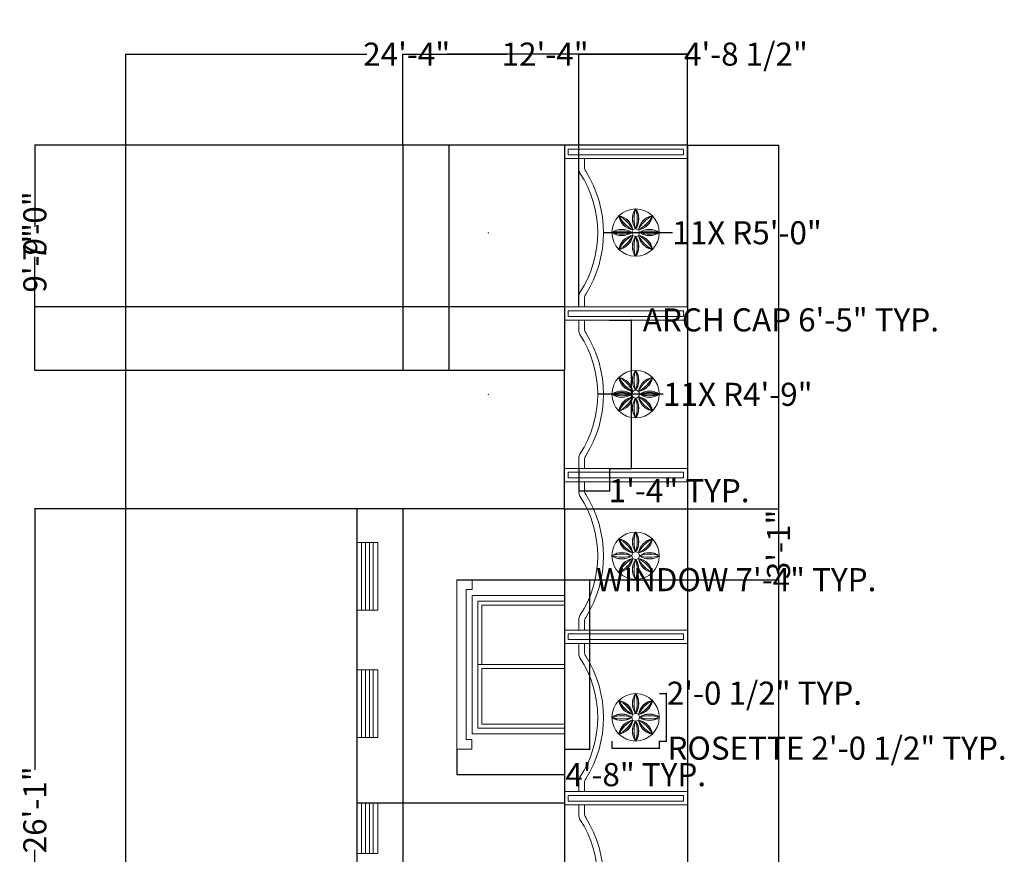
# Model space of a CAD drawing. Units: inches. Extents: x 1146 to 2917, y 889 to 2437.
# Tile 13 of 13: x 2405 to 2917, y 2003 to 2437. Entities that reach past the tile are written whole.
import ezdxf

# ---------------------------------------------------------------- set-up
doc = ezdxf.new("R2010")
doc.units = ezdxf.units.IN
doc.header["$MEASUREMENT"] = 0
for name, color, linetype, lineweight in [('A-ANNO-DIMS', 2, 'Continuous', 18), ('A-ELEV', 7, 'Continuous', 30), ('A-ELEV-GLAZ', 5, 'Continuous', 18), ('A-ELEV-ORNM', 8, 'Continuous', 18)]:
    doc.layers.add(name, color=color, linetype=linetype, lineweight=lineweight)
doc.styles.get("Standard").update_dxf_attribs({"font": 'arial.ttf'})
doc.dimstyles.get("Standard").update_dxf_attribs({"dimtxt": 12, "dimasz": 0.18, "dimexe": 0.18, "dimexo": 0.0625, "dimgap": 0.09, "dimtad": 0, "dimtoh": 1, "dimdec": 1, "dimzin": 0, "dimdsep": 46, "dimlunit": 4, "dimtxsty": 'Standard', "dimcen": 0.09, "dimadec": 0, "dimazin": 0, "dimtfac": 1, "dimtdec": 1, "dimtofl": 0, "dimtmove": 0, "dimatfit": 3, "dimfxl": 1, "dimtolj": 1, "dimtzin": 0, "dimarcsym": 0})

# ---------------------------------------------------------------- blocks, each defined once
blk = doc.blocks.new('BOUNDARY-WALL-PIER')
for points in [[(0, 6.94), (64, 6.94), (64, 0), (0, 0)], [(2, 4.94), (62, 4.94), (62, 2), (2, 2)]]:
    blk.add_lwpolyline(points, close=True)
blk = doc.blocks.new('PARAPET-LOUVER')
for p, q in [((2.58, 0), (2.58, 35.13)), ((4.58, 0), (4.58, 35.13)), ((6.58, 0), (6.58, 35.13)), ((8.58, 0), (8.58, 35.13))]:
    blk.add_line(p, q)
blk.add_lwpolyline([(0, 0), (11.07, 0), (11.07, 35.13), (0, 35.13)], close=True)
blk = doc.blocks.new('WINDOW-ELEV-72')
for p, q in [((8, 83), (8, 88)), ((11, 44), (11, 77)), ((11, 77), (56, 77)), ((11, 11), (11, 44)), ((56, 44), (11, 44)), ((56, 11), (11, 11)), ((7.96, 5), (7.96, 0))]:
    blk.add_line(p, q)
for points in [[(7.96, 0), (0, 0), (0, 88), (8, 88)], [(7.96, 5), (5, 5), (5, 83), (8, 83)], [(56, 8), (8, 8), (8, 80), (56, 80)], [(13, 44), (13, 75), (56, 75)], [(13, 42), (56, 42)], [(56, 13), (13, 13), (13, 42)]]:
    blk.add_lwpolyline(points)
blk = doc.blocks.new('BOUNDARY-WALL-ARCH-CAP')
for p, q in [((0, 71.74), (0, 77.06)), ((3, 72.62), (3, 77.06)), ((0, 0), (0, 5.32)), ((3, 0), (3, 4.44))]:
    blk.add_line(p, q)
for centre, radius, start, end in [((4, 71.74), 4, 180, 213.079), ((7, 72.62), 4, 180, 212.2708), ((-46.98, 38.53), 56.85, 326.921, 33.079), ((-46.98, 38.53), 59.85, 327.7292, 32.2708), ((4, 5.32), 4, 146.921, 180), ((7, 4.44), 4, 147.7292, 180)]:
    blk.add_arc(centre, radius, start, end)
blk = doc.blocks.new('ROSETTE-PLANAR-TRACERY')
for radius in [12.33, 2.02]:
    blk.add_circle((12.33, 12.33), radius)
for centre, radius, start, end in [((2.21, 12.37), 8.8, 9.1552, 80.8448), ((12.65, 22.8), 9.21, 190.95, 259.05), ((19.96, 19.51), 9.21, 145.95, 214.05), ((5.2, 19.51), 8.8, 324.1552, 35.8448), ((12.37, 22.46), 8.8, 279.1552, 350.8448), ((22.8, 12.02), 9.21, 100.95, 169.05), ((5.15, 5.2), 8.8, 54.1552, 125.8448), ((5.15, 19.96), 9.21, 235.95, 304.05), ((12.3, 2.21), 8.8, 99.1552, 170.8448), ((1.86, 12.65), 9.21, 280.95, 349.05), ((19.47, 5.15), 8.8, 144.1552, 215.8448), ((4.71, 5.15), 9.21, 325.95, 34.05), ((22.46, 12.3), 8.8, 189.1552, 260.8448), ((12.02, 1.86), 9.21, 10.95, 79.05), ((19.51, 4.71), 9.21, 55.95, 124.05), ((19.51, 19.47), 8.8, 234.1552, 305.8448)]:
    blk.add_arc(centre, radius, start, end)
at = {"extrusion": (-2e-16, -2e-16, -1)}
for centre, radius, start, end in [((-12.3, 22.46), 8.8, 279.1552, 350.8448), ((-1.86, 12.02), 9.21, 100.95, 169.05)]:
    blk.add_arc(centre, radius, start, end, dxfattribs=at)
at = {"extrusion": (-2e-16, 0, -1)}
for centre, radius, start, end in [((-19.47, 19.51), 8.8, 324.1552, 35.8448), ((-4.71, 19.51), 9.21, 145.95, 214.05)]:
    blk.add_arc(centre, radius, start, end, dxfattribs=at)
at = {"extrusion": (-2e-16, 2e-16, -1)}
for centre, radius, start, end in [((-22.46, 12.37), 8.8, 9.1552, 80.8448), ((-12.02, 22.8), 9.21, 190.95, 259.05)]:
    blk.add_arc(centre, radius, start, end, dxfattribs=at)
at = {"extrusion": (0, -2e-16, -1)}
for centre, radius, start, end in [((-5.15, 4.71), 9.21, 55.95, 124.05), ((-5.15, 19.47), 8.8, 234.1552, 305.8448)]:
    blk.add_arc(centre, radius, start, end, dxfattribs=at)
at = {"extrusion": (2e-16, -2e-16, -1)}
for centre, radius, start, end in [((-2.21, 12.3), 8.8, 189.1552, 260.8448), ((-12.65, 1.86), 9.21, 10.95, 79.05)]:
    blk.add_arc(centre, radius, start, end, dxfattribs=at)
at = {"extrusion": (2e-16, 0, -1)}
for centre, radius, start, end in [((-19.96, 5.15), 9.21, 325.95, 34.05), ((-5.2, 5.15), 8.8, 144.1552, 215.8448)]:
    blk.add_arc(centre, radius, start, end, dxfattribs=at)
at = {"extrusion": (2e-16, 2e-16, -1)}
for centre, radius, start, end in [((-12.37, 2.21), 8.8, 99.1552, 170.8448), ((-22.8, 12.65), 9.21, 280.95, 349.05)]:
    blk.add_arc(centre, radius, start, end, dxfattribs=at)
at = {"extrusion": (0, 2e-16, -1)}
for centre, radius, start, end in [((-19.51, 5.2), 8.8, 54.1552, 125.8448), ((-19.51, 19.96), 9.21, 235.95, 304.05)]:
    blk.add_arc(centre, radius, start, end, dxfattribs=at)
blk = doc.blocks.new('*D85')
at = {"layer": 'A-ANNO-DIMS', "color": 0, "lineweight": -2, "transparency": 16777216}
for p, q in [((2711.67, 2280.45), (2723.35, 2280.45)), ((2723.17, 2280.45), (2723.17, 2280.63)), ((2723.17, 2280.63), (2723.35, 2280.63)), ((2723.17, 2203.57), (2723.17, 2280.27)), ((2711.67, 2203.39), (2723.35, 2203.39))]:
    blk.add_line(p, q, dxfattribs=at)
at = {"layer": 'A-ANNO-DIMS', "color": 0, "transparency": 16777216}
for points in [[(2723.14, 2280.27), (2723.2, 2280.27), (2723.17, 2280.45)], [(2723.14, 2203.57), (2723.2, 2203.57), (2723.17, 2203.39)]]:
    blk.add_solid(points, dxfattribs=at)
at = {"layer": 'Defpoints', "color": 0, "transparency": 16777216}
for p in [(2711.61, 2280.45), (2723.17, 2280.45), (2711.61, 2203.39)]:
    blk.add_point(p, dxfattribs=at)
at = {"layer": 'A-ANNO-DIMS', "color": 0, "transparency": 16777216, "insert": (2806, 2280.63), "char_height": 12, "attachment_point": 5}
blk.add_mtext('\\A1;ARCH CAP 6\'-5" TYP.', dxfattribs=at)
blk = doc.blocks.new('*D86')
at = {"layer": 'A-ANNO-DIMS', "color": 0, "lineweight": -2, "transparency": 16777216}
for p, q in [((2695.67, 2203.33), (2695.67, 2191.65)), ((2711.61, 2203.33), (2711.61, 2191.65)), ((2695.85, 2191.83), (2711.43, 2191.83)), ((2711.61, 2191.83), (2711.79, 2191.83))]:
    blk.add_line(p, q, dxfattribs=at)
at = {"layer": 'A-ANNO-DIMS', "color": 0, "transparency": 16777216}
for points in [[(2695.85, 2191.86), (2695.85, 2191.8), (2695.67, 2191.83)], [(2711.43, 2191.86), (2711.43, 2191.8), (2711.61, 2191.83)]]:
    blk.add_solid(points, dxfattribs=at)
at = {"layer": 'Defpoints', "color": 0, "transparency": 16777216}
for p in [(2695.67, 2203.39), (2711.61, 2203.39), (2711.61, 2191.83)]:
    blk.add_point(p, dxfattribs=at)
at = {"layer": 'A-ANNO-DIMS', "color": 0, "transparency": 16777216, "insert": (2747.89, 2191.83), "char_height": 12, "attachment_point": 5}
blk.add_mtext('\\A1;1\'-4" TYP.', dxfattribs=at)
blk = doc.blocks.new('*D87')
at = {"layer": 'A-ANNO-DIMS', "color": 0, "lineweight": -2, "transparency": 16777216}
for p, q in [((2712.92, 2061.61), (2712.92, 2057.79)), ((2737.59, 2061.61), (2737.59, 2057.79)), ((2713.1, 2057.97), (2737.41, 2057.97)), ((2737.59, 2057.97), (2737.77, 2057.97))]:
    blk.add_line(p, q, dxfattribs=at)
at = {"layer": 'A-ANNO-DIMS', "color": 0, "transparency": 16777216}
for points in [[(2713.1, 2058), (2713.1, 2057.94), (2712.92, 2057.97)], [(2737.41, 2058), (2737.41, 2057.94), (2737.59, 2057.97)]]:
    blk.add_solid(points, dxfattribs=at)
at = {"layer": 'Defpoints', "color": 0, "transparency": 16777216}
for p in [(2712.92, 2061.67), (2737.59, 2061.67), (2737.59, 2057.97)]:
    blk.add_point(p, dxfattribs=at)
at = {"layer": 'A-ANNO-DIMS', "color": 0, "transparency": 16777216, "insert": (2830.02, 2057.97), "char_height": 12, "attachment_point": 5}
blk.add_mtext('\\A1;ROSETTE 2\'-0 1/2" TYP.', dxfattribs=at)
blk = doc.blocks.new('*D88')
at = {"layer": 'A-ANNO-DIMS', "color": 0, "lineweight": -2, "transparency": 16777216}
for p, q in [((2737.65, 2086.34), (2741.47, 2086.34)), ((2741.29, 2086.34), (2741.29, 2086.52)), ((2741.29, 2086.52), (2741.47, 2086.52)), ((2741.29, 2061.85), (2741.29, 2086.16)), ((2737.65, 2061.67), (2741.47, 2061.67))]:
    blk.add_line(p, q, dxfattribs=at)
at = {"layer": 'A-ANNO-DIMS', "color": 0, "transparency": 16777216}
for points in [[(2741.26, 2086.16), (2741.32, 2086.16), (2741.29, 2086.34)], [(2741.26, 2061.85), (2741.32, 2061.85), (2741.29, 2061.67)]]:
    blk.add_solid(points, dxfattribs=at)
at = {"layer": 'Defpoints', "color": 0, "transparency": 16777216}
for p in [(2737.59, 2086.34), (2741.29, 2086.34), (2737.59, 2061.67)]:
    blk.add_point(p, dxfattribs=at)
at = {"layer": 'A-ANNO-DIMS', "color": 0, "transparency": 16777216, "insert": (2792.22, 2086.52), "char_height": 12, "attachment_point": 5}
blk.add_mtext('\\A1;2\'-0 1/2" TYP.', dxfattribs=at)
blk = doc.blocks.new('*D91')
at = {"layer": 'A-ANNO-DIMS', "color": 0, "lineweight": -2, "transparency": 16777216}
for p, q in [((2688.26, 2145.39), (2701.58, 2145.39)), ((2701.4, 2145.39), (2701.4, 2145.57)), ((2701.4, 2145.57), (2701.58, 2145.57)), ((2701.4, 2057.57), (2701.4, 2145.21)), ((2688.26, 2057.39), (2701.58, 2057.39))]:
    blk.add_line(p, q, dxfattribs=at)
at = {"layer": 'A-ANNO-DIMS', "color": 0, "transparency": 16777216}
for points in [[(2701.37, 2145.21), (2701.43, 2145.21), (2701.4, 2145.39)], [(2701.37, 2057.57), (2701.43, 2057.57), (2701.4, 2057.39)]]:
    blk.add_solid(points, dxfattribs=at)
at = {"layer": 'Defpoints', "color": 0, "transparency": 16777216}
for p in [(2688.2, 2145.39), (2701.4, 2145.39), (2688.2, 2057.39)]:
    blk.add_point(p, dxfattribs=at)
at = {"layer": 'A-ANNO-DIMS', "color": 0, "transparency": 16777216, "insert": (2777.6, 2145.57), "char_height": 12, "attachment_point": 5}
blk.add_mtext('\\A1;WINDOW 7\'-4" TYP.', dxfattribs=at)
blk = doc.blocks.new('*D92')
at = {"layer": 'A-ANNO-DIMS', "color": 0, "lineweight": -2, "transparency": 16777216}
for p, q in [((2632.2, 2057.33), (2632.2, 2044.01)), ((2688.2, 2057.33), (2688.2, 2044.01)), ((2632.38, 2044.19), (2688.02, 2044.19)), ((2688.2, 2044.19), (2688.38, 2044.19))]:
    blk.add_line(p, q, dxfattribs=at)
at = {"layer": 'A-ANNO-DIMS', "color": 0, "transparency": 16777216}
for points in [[(2632.38, 2044.22), (2632.38, 2044.16), (2632.2, 2044.19)], [(2688.02, 2044.22), (2688.02, 2044.16), (2688.2, 2044.19)]]:
    blk.add_solid(points, dxfattribs=at)
at = {"layer": 'Defpoints', "color": 0, "transparency": 16777216}
for p in [(2632.2, 2057.39), (2688.2, 2057.39), (2688.2, 2044.19)]:
    blk.add_point(p, dxfattribs=at)
at = {"layer": 'A-ANNO-DIMS', "color": 0, "transparency": 16777216, "insert": (2725.29, 2044.19), "char_height": 12, "attachment_point": 5}
blk.add_mtext('\\A1;4\'-8" TYP.', dxfattribs=at)
blk = doc.blocks.new('*D121')
at = {"layer": 'A-ANNO-DIMS', "color": 0, "lineweight": -2, "transparency": 16777216}
for p, q in [((2752.26, 2371.39), (2799.78, 2371.39)), ((2799.6, 2371.21), (2799.6, 1936.27)), ((2799.6, 1432.07), (2799.6, 1867.01)), ((2752.26, 1431.89), (2799.78, 1431.89))]:
    blk.add_line(p, q, dxfattribs=at)
at = {"layer": 'A-ANNO-DIMS', "color": 0, "transparency": 16777216}
for points in [[(2799.57, 2371.21), (2799.63, 2371.21), (2799.6, 2371.39)], [(2799.57, 1432.07), (2799.63, 1432.07), (2799.6, 1431.89)]]:
    blk.add_solid(points, dxfattribs=at)
at = {"layer": 'Defpoints', "color": 0, "transparency": 16777216}
for p in [(2752.2, 2371.39), (2799.6, 2371.39), (2752.2, 1431.89)]:
    blk.add_point(p, dxfattribs=at)
at = {"layer": 'A-ANNO-DIMS', "color": 0, "transparency": 16777216, "insert": (2799.6, 1901.64), "char_height": 12, "attachment_point": 5, "rotation": 90}
blk.add_mtext('\\A1;78\'-3 1/2"', dxfattribs=at)
blk = doc.blocks.new('*D122')
at = {"layer": 'A-ANNO-DIMS', "color": 0, "lineweight": -2, "transparency": 16777216}
for p, q in [((2460.2, 1869.45), (2460.2, 2418.97)), ((2460.38, 2418.79), (2585.4, 2418.79)), ((2752.02, 2418.79), (2627, 2418.79)), ((2752.2, 2371.45), (2752.2, 2418.97))]:
    blk.add_line(p, q, dxfattribs=at)
at = {"layer": 'A-ANNO-DIMS', "color": 0, "transparency": 16777216}
for points in [[(2460.38, 2418.82), (2460.38, 2418.76), (2460.2, 2418.79)], [(2752.02, 2418.82), (2752.02, 2418.76), (2752.2, 2418.79)]]:
    blk.add_solid(points, dxfattribs=at)
at = {"layer": 'Defpoints', "color": 0, "transparency": 16777216}
for p in [(2752.2, 2418.79), (2752.2, 2371.39), (2460.2, 1869.39)]:
    blk.add_point(p, dxfattribs=at)
at = {"layer": 'A-ANNO-DIMS', "color": 0, "transparency": 16777216, "insert": (2606.2, 2418.79), "char_height": 12, "attachment_point": 5}
blk.add_mtext('\\A1;24\'-4"', dxfattribs=at)
blk = doc.blocks.new('*D123')
at = {"layer": 'A-ANNO-DIMS', "color": 0, "lineweight": -2, "transparency": 16777216}
for p, q in [((2688.14, 2371.39), (2412.62, 2371.39)), ((2412.8, 2371.21), (2412.8, 2345.38)), ((2412.8, 2287.57), (2412.8, 2313.4)), ((2688.14, 2287.39), (2412.62, 2287.39))]:
    blk.add_line(p, q, dxfattribs=at)
at = {"layer": 'A-ANNO-DIMS', "color": 0, "transparency": 16777216}
for points in [[(2412.77, 2371.21), (2412.83, 2371.21), (2412.8, 2371.39)], [(2412.77, 2287.57), (2412.83, 2287.57), (2412.8, 2287.39)]]:
    blk.add_solid(points, dxfattribs=at)
at = {"layer": 'Defpoints', "color": 0, "transparency": 16777216}
for p in [(2412.8, 2371.39), (2688.2, 2371.39), (2688.2, 2287.39)]:
    blk.add_point(p, dxfattribs=at)
at = {"layer": 'A-ANNO-DIMS', "color": 0, "transparency": 16777216, "insert": (2412.8, 2329.39), "char_height": 12, "attachment_point": 5, "rotation": 90}
blk.add_mtext('\\A1;7\'-0"', dxfattribs=at)
blk = doc.blocks.new('*D124')
at = {"layer": 'A-ANNO-DIMS', "color": 0, "lineweight": -2, "transparency": 16777216}
for p, q in [((2695.67, 2287.45), (2695.67, 2418.97)), ((2695.85, 2418.79), (2752.02, 2418.79)), ((2752.2, 2287.45), (2752.2, 2418.97)), ((2752.2, 2418.79), (2752.38, 2418.79))]:
    blk.add_line(p, q, dxfattribs=at)
at = {"layer": 'A-ANNO-DIMS', "color": 0, "transparency": 16777216}
for points in [[(2695.85, 2418.82), (2695.85, 2418.76), (2695.67, 2418.79)], [(2752.02, 2418.82), (2752.02, 2418.76), (2752.2, 2418.79)]]:
    blk.add_solid(points, dxfattribs=at)
at = {"layer": 'Defpoints', "color": 0, "transparency": 16777216}
for p in [(2752.2, 2418.79), (2695.67, 2287.39), (2752.2, 2287.39)]:
    blk.add_point(p, dxfattribs=at)
at = {"layer": 'A-ANNO-DIMS', "color": 0, "transparency": 16777216, "insert": (2782.64, 2418.79), "char_height": 12, "attachment_point": 5}
blk.add_mtext('\\A1;4\'-8 1/2"', dxfattribs=at)
blk = doc.blocks.new('*D127')
at = {"layer": 'A-ANNO-DIMS', "color": 0, "lineweight": -2, "transparency": 16777216}
for p, q in [((2580.14, 2182.39), (2412.62, 2182.39)), ((2412.8, 2182.21), (2412.8, 2046.7)), ((2412.8, 1869.57), (2412.8, 2005.09)), ((2460.14, 1869.39), (2412.62, 1869.39))]:
    blk.add_line(p, q, dxfattribs=at)
at = {"layer": 'A-ANNO-DIMS', "color": 0, "transparency": 16777216}
for points in [[(2412.77, 2182.21), (2412.83, 2182.21), (2412.8, 2182.39)], [(2412.77, 1869.57), (2412.83, 1869.57), (2412.8, 1869.39)]]:
    blk.add_solid(points, dxfattribs=at)
at = {"layer": 'Defpoints', "color": 0, "transparency": 16777216}
for p in [(2412.8, 2182.39), (2580.2, 2182.39), (2460.2, 1869.39)]:
    blk.add_point(p, dxfattribs=at)
at = {"layer": 'A-ANNO-DIMS', "color": 0, "transparency": 16777216, "insert": (2412.8, 2025.89), "char_height": 12, "attachment_point": 5, "rotation": 90}
blk.add_mtext('\\A1;26\'-1"', dxfattribs=at)
blk = doc.blocks.new('*D136')
at = {"layer": 'A-ANNO-DIMS', "color": 0, "lineweight": -2, "transparency": 16777216}
for p, q in [((2604.2, 2371.45), (2604.2, 2418.97)), ((2604.38, 2418.79), (2658.06, 2418.79)), ((2752.02, 2418.79), (2698.34, 2418.79)), ((2752.2, 2371.45), (2752.2, 2418.97))]:
    blk.add_line(p, q, dxfattribs=at)
at = {"layer": 'A-ANNO-DIMS', "color": 0, "transparency": 16777216}
for points in [[(2604.38, 2418.82), (2604.38, 2418.76), (2604.2, 2418.79)], [(2752.02, 2418.82), (2752.02, 2418.76), (2752.2, 2418.79)]]:
    blk.add_solid(points, dxfattribs=at)
at = {"layer": 'Defpoints', "color": 0, "transparency": 16777216}
for p in [(2604.2, 2418.79), (2604.2, 2371.39), (2752.2, 2371.39)]:
    blk.add_point(p, dxfattribs=at)
at = {"layer": 'A-ANNO-DIMS', "color": 0, "transparency": 16777216, "insert": (2678.2, 2418.79), "char_height": 12, "attachment_point": 5}
blk.add_mtext('\\A1;12\'-4"', dxfattribs=at)
blk = doc.blocks.new('*D137')
at = {"layer": 'A-ANNO-DIMS', "color": 0, "lineweight": -2, "transparency": 16777216}
for p, q in [((2604.14, 2371.39), (2412.62, 2371.39)), ((2412.8, 2371.21), (2412.8, 2328.93)), ((2412.8, 2254.57), (2412.8, 2296.85)), ((2604.14, 2254.39), (2412.62, 2254.39))]:
    blk.add_line(p, q, dxfattribs=at)
at = {"layer": 'A-ANNO-DIMS', "color": 0, "transparency": 16777216}
for points in [[(2412.77, 2371.21), (2412.83, 2371.21), (2412.8, 2371.39)], [(2412.77, 2254.57), (2412.83, 2254.57), (2412.8, 2254.39)]]:
    blk.add_solid(points, dxfattribs=at)
at = {"layer": 'Defpoints', "color": 0, "transparency": 16777216}
for p in [(2604.2, 2371.39), (2412.8, 2254.39), (2604.2, 2254.39)]:
    blk.add_point(p, dxfattribs=at)
at = {"layer": 'A-ANNO-DIMS', "color": 0, "transparency": 16777216, "insert": (2412.8, 2312.89), "char_height": 12, "attachment_point": 5, "rotation": 90}
blk.add_mtext('\\A1;9\'-9"', dxfattribs=at)
blk = doc.blocks.new('*D140')
at = {"layer": 'A-ANNO-DIMS', "color": 0, "lineweight": -2, "transparency": 16777216}
for p, q in [((2688.26, 2182.39), (2799.78, 2182.39)), ((2799.6, 2182.21), (2799.6, 2179.93)), ((2799.6, 2145.57), (2799.6, 2147.86)), ((2632.26, 2145.39), (2799.78, 2145.39))]:
    blk.add_line(p, q, dxfattribs=at)
at = {"layer": 'A-ANNO-DIMS', "color": 0, "transparency": 16777216}
for points in [[(2799.57, 2182.21), (2799.63, 2182.21), (2799.6, 2182.39)], [(2799.57, 2145.57), (2799.63, 2145.57), (2799.6, 2145.39)]]:
    blk.add_solid(points, dxfattribs=at)
at = {"layer": 'Defpoints', "color": 0, "transparency": 16777216}
for p in [(2688.2, 2182.39), (2632.2, 2145.39), (2799.6, 2145.39)]:
    blk.add_point(p, dxfattribs=at)
at = {"layer": 'A-ANNO-DIMS', "color": 0, "transparency": 16777216, "insert": (2799.6, 2163.89), "char_height": 12, "attachment_point": 5, "rotation": 90}
blk.add_mtext('\\A1;3\'-1"', dxfattribs=at)
blk = doc.blocks.new('*D172')
at = {"layer": 'A-ANNO-DIMS', "color": 0, "lineweight": -2, "transparency": 16777216}
for p, q in [((2648.59, 2325.92), (2648.77, 2325.92)), ((2648.68, 2325.83), (2648.68, 2326.01)), ((2744.44, 2325.92), (2708.71, 2325.92))]:
    blk.add_line(p, q, dxfattribs=at)
at = {"layer": 'A-ANNO-DIMS', "color": 0, "transparency": 16777216}
blk.add_solid([(2708.71, 2325.95), (2708.71, 2325.89), (2708.53, 2325.92)], dxfattribs=at)
at = {"layer": 'Defpoints', "color": 0, "transparency": 16777216}
for p in [(2648.68, 2325.92), (2708.53, 2325.92)]:
    blk.add_point(p, dxfattribs=at)
at = {"layer": 'A-ANNO-DIMS', "color": 0, "transparency": 16777216, "insert": (2783.21, 2325.92), "char_height": 12, "attachment_point": 5}
blk.add_mtext('\\A1;11X R5\'-0"', dxfattribs=at)
blk = doc.blocks.new('*D173')
at = {"layer": 'A-ANNO-DIMS', "color": 0, "lineweight": -2, "transparency": 16777216}
for p, q in [((2648.59, 2241.92), (2648.77, 2241.92)), ((2648.68, 2241.83), (2648.68, 2242.01)), ((2739.64, 2241.92), (2705.71, 2241.92))]:
    blk.add_line(p, q, dxfattribs=at)
at = {"layer": 'A-ANNO-DIMS', "color": 0, "transparency": 16777216}
blk.add_solid([(2705.71, 2241.95), (2705.71, 2241.89), (2705.53, 2241.92)], dxfattribs=at)
at = {"layer": 'Defpoints', "color": 0, "transparency": 16777216}
for p in [(2648.68, 2241.92), (2705.53, 2241.92)]:
    blk.add_point(p, dxfattribs=at)
at = {"layer": 'A-ANNO-DIMS', "color": 0, "transparency": 16777216, "insert": (2778.41, 2241.92), "char_height": 12, "attachment_point": 5}
blk.add_mtext('\\A1;11X R4\'-9"', dxfattribs=at)

msp = doc.modelspace()

# ---------------------------------------------------------------- linework, layer by layer
at = {"layer": 'A-ELEV'}
for p, q in [((2752.2, 2371.39), (2604.2, 2371.39)), ((2604.2, 2371.39), (2604.2, 2254.39)), ((2628.2, 2371.39), (2628.2, 2254.39)), ((2688.2, 2371.39), (2688.2, 2254.39)), ((2752.2, 2371.39), (2752.2, 1431.89)), ((2688.2, 2254.39), (2604.2, 2254.39)), ((2688.2, 2182.39), (2688.2, 2254.39)), ((2688.2, 2182.39), (2580.2, 2182.39)), ((2580.2, 2182.39), (2580.2, 1869.39)), ((2604.2, 2182.39), (2604.2, 1869.39)), ((2688.2, 2182.39), (2688.2, 1431.89)), ((2688.2, 2029.39), (2580.2, 2029.39))]:
    msp.add_line(p, q, dxfattribs=at)
at = {"layer": 'A-ELEV-ORNM'}
for p, q in [((2582.78, 2003.23), (2582.78, 2029.39)), ((2584.78, 2003.23), (2584.78, 2029.39)), ((2586.78, 2003.23), (2586.78, 2029.39)), ((2588.78, 2003.23), (2588.78, 2029.39))]:
    msp.add_line(p, q, dxfattribs=at)
msp.add_lwpolyline([(2580.2, 2038.36), (2580.2, 2003.23), (2591.27, 2003.23), (2591.27, 2029.39)], dxfattribs=at)
at = {"layer": 'A-ELEV-ORNM', "extrusion": (0.866025, 5.48447e-11, -0.5)}
for centre, radius, start, end in [((2333.18, 1369.76, 2360.14), 8.8, 234.1552, 305.8448), ((2333.18, 1355, 2360.14), 9.21, 55.95, 124.05), ((2249.18, 1369.76, 2360.14), 8.8, 234.1552, 305.8448), ((2249.18, 1355, 2360.14), 9.21, 55.95, 124.05), ((2165.18, 1369.76, 2360.14), 8.8, 234.1552, 305.8448), ((2165.18, 1355, 2360.14), 9.21, 55.95, 124.05), ((2081.18, 1369.76, 2360.14), 8.8, 234.1552, 305.8448), ((2081.18, 1355, 2360.14), 9.21, 55.95, 124.05)]:
    msp.add_arc(centre, radius, start, end, dxfattribs=at)
at = {"layer": 'A-ELEV-ORNM', "extrusion": (-0.866025, -5.48447e-11, -0.5)}
for centre, radius, start, end in [((-2333.18, -1369.76, -2360.14), 8.8, 54.1552, 125.8448), ((-2333.18, -1355, -2360.14), 9.21, 235.95, 304.05), ((-2249.18, -1369.76, -2360.14), 8.8, 54.1552, 125.8448), ((-2249.18, -1355, -2360.14), 9.21, 235.95, 304.05), ((-2165.18, -1369.76, -2360.14), 8.8, 54.1552, 125.8448), ((-2165.18, -1355, -2360.14), 9.21, 235.95, 304.05), ((-2081.18, -1369.76, -2360.14), 8.8, 54.1552, 125.8448), ((-2081.18, -1355, -2360.14), 9.21, 235.95, 304.05)]:
    msp.add_arc(centre, radius, start, end, dxfattribs=at)
at = {"layer": 'A-ELEV-ORNM', "extrusion": (0.866025, 5.48447e-11, 0.5)}
for centre, radius, start, end in [((2333.18, -1370.26, 2360.14), 9.21, 55.95, 124.05), ((2333.18, -1355.49, 2360.14), 8.8, 234.1552, 305.8448), ((2249.18, -1370.26, 2360.14), 9.21, 55.95, 124.05), ((2249.18, -1355.49, 2360.14), 8.8, 234.1552, 305.8448), ((2165.18, -1370.26, 2360.14), 9.21, 55.95, 124.05), ((2165.18, -1355.49, 2360.14), 8.8, 234.1552, 305.8448), ((2081.18, -1370.26, 2360.14), 9.21, 55.95, 124.05), ((2081.18, -1355.49, 2360.14), 8.8, 234.1552, 305.8448)]:
    msp.add_arc(centre, radius, start, end, dxfattribs=at)
at = {"layer": 'A-ELEV-ORNM', "extrusion": (-0.866025, -5.48447e-11, 0.5)}
for centre, radius, start, end in [((-2333.18, 1370.26, -2360.14), 9.21, 235.95, 304.05), ((-2333.18, 1355.49, -2360.14), 8.8, 54.1552, 125.8448), ((-2249.18, 1370.26, -2360.14), 9.21, 235.95, 304.05), ((-2249.18, 1355.49, -2360.14), 8.8, 54.1552, 125.8448), ((-2165.18, 1370.26, -2360.14), 9.21, 235.95, 304.05), ((-2165.18, 1355.49, -2360.14), 8.8, 54.1552, 125.8448), ((-2081.18, 1370.26, -2360.14), 9.21, 235.95, 304.05), ((-2081.18, 1355.49, -2360.14), 8.8, 54.1552, 125.8448)]:
    msp.add_arc(centre, radius, start, end, dxfattribs=at)
at = {"layer": 'A-ELEV-ORNM', "extrusion": (0.612372, 0.612372, 0.5)}
for centre, radius, start, end in [((-275.14, -1778.75, 3093.25), 8.8, 234.1552, 305.8448), ((-275.14, -1793.52, 3093.25), 9.21, 55.95, 124.05), ((-289.49, -1793.02, 3093.25), 8.8, 54.1552, 125.8448), ((-289.49, -1778.26, 3093.25), 9.21, 235.95, 304.05), ((-334.53, -1749.06, 3041.81), 8.8, 234.1552, 305.8448), ((-334.53, -1763.82, 3041.81), 9.21, 55.95, 124.05), ((-348.89, -1763.33, 3041.81), 8.8, 54.1552, 125.8448), ((-348.89, -1748.56, 3041.81), 9.21, 235.95, 304.05), ((-393.93, -1719.36, 2990.37), 8.8, 234.1552, 305.8448), ((-393.93, -1734.12, 2990.37), 9.21, 55.95, 124.05), ((-408.29, -1733.63, 2990.37), 8.8, 54.1552, 125.8448), ((-408.29, -1718.87, 2990.37), 9.21, 235.95, 304.05), ((-453.33, -1689.66, 2938.93), 8.8, 234.1552, 305.8448), ((-453.33, -1704.42, 2938.93), 9.21, 55.95, 124.05), ((-467.68, -1703.93, 2938.93), 8.8, 54.1552, 125.8448), ((-467.68, -1689.17, 2938.93), 9.21, 235.95, 304.05)]:
    msp.add_arc(centre, radius, start, end, dxfattribs=at)
at = {"layer": 'A-ELEV-ORNM', "extrusion": (0.612372, 0.612372, -0.5)}
for centre, radius, start, end in [((-275.14, 1793.02, 3093.25), 8.8, 234.1552, 305.8448), ((-275.14, 1778.26, 3093.25), 9.21, 55.95, 124.05), ((-289.49, 1778.75, 3093.25), 8.8, 54.1552, 125.8448), ((-289.49, 1793.52, 3093.25), 9.21, 235.95, 304.05), ((-334.53, 1763.33, 3041.81), 8.8, 234.1552, 305.8448), ((-334.53, 1748.56, 3041.81), 9.21, 55.95, 124.05), ((-348.89, 1749.06, 3041.81), 8.8, 54.1552, 125.8448), ((-348.89, 1763.82, 3041.81), 9.21, 235.95, 304.05), ((-393.93, 1733.63, 2990.37), 8.8, 234.1552, 305.8448), ((-393.93, 1718.87, 2990.37), 9.21, 55.95, 124.05), ((-408.29, 1719.36, 2990.37), 8.8, 54.1552, 125.8448), ((-408.29, 1734.12, 2990.37), 9.21, 235.95, 304.05), ((-453.33, 1703.93, 2938.93), 8.8, 234.1552, 305.8448), ((-453.33, 1689.17, 2938.93), 9.21, 55.95, 124.05), ((-467.68, 1689.66, 2938.93), 8.8, 54.1552, 125.8448), ((-467.68, 1704.42, 2938.93), 9.21, 235.95, 304.05)]:
    msp.add_arc(centre, radius, start, end, dxfattribs=at)
at = {"layer": 'A-ELEV-ORNM', "extrusion": (-0.612372, -0.612372, -0.5)}
for centre, radius, start, end in [((275.14, -1793.02, -3093.25), 8.8, 54.1552, 125.8448), ((275.14, -1778.26, -3093.25), 9.21, 235.95, 304.05), ((289.49, -1778.75, -3093.25), 8.8, 234.1552, 305.8448), ((289.49, -1793.52, -3093.25), 9.21, 55.95, 124.05), ((334.53, -1763.33, -3041.81), 8.8, 54.1552, 125.8448), ((334.53, -1748.56, -3041.81), 9.21, 235.95, 304.05), ((348.89, -1749.06, -3041.81), 8.8, 234.1552, 305.8448), ((348.89, -1763.82, -3041.81), 9.21, 55.95, 124.05), ((393.93, -1733.63, -2990.37), 8.8, 54.1552, 125.8448), ((393.93, -1718.87, -2990.37), 9.21, 235.95, 304.05), ((408.29, -1719.36, -2990.37), 8.8, 234.1552, 305.8448), ((408.29, -1734.12, -2990.37), 9.21, 55.95, 124.05), ((453.33, -1703.93, -2938.93), 8.8, 54.1552, 125.8448), ((453.33, -1689.17, -2938.93), 9.21, 235.95, 304.05), ((467.68, -1689.66, -2938.93), 8.8, 234.1552, 305.8448), ((467.68, -1704.42, -2938.93), 9.21, 55.95, 124.05)]:
    msp.add_arc(centre, radius, start, end, dxfattribs=at)
at = {"layer": 'A-ELEV-ORNM', "extrusion": (-0.612372, -0.612372, 0.5)}
for centre, radius, start, end in [((275.14, 1778.75, -3093.25), 8.8, 54.1552, 125.8448), ((275.14, 1793.52, -3093.25), 9.21, 235.95, 304.05), ((289.49, 1793.02, -3093.25), 8.8, 234.1552, 305.8448), ((289.49, 1778.26, -3093.25), 9.21, 55.95, 124.05), ((334.53, 1749.06, -3041.81), 8.8, 54.1552, 125.8448), ((334.53, 1763.82, -3041.81), 9.21, 235.95, 304.05), ((348.89, 1763.33, -3041.81), 8.8, 234.1552, 305.8448), ((348.89, 1748.56, -3041.81), 9.21, 55.95, 124.05), ((393.93, 1719.36, -2990.37), 8.8, 54.1552, 125.8448), ((393.93, 1734.12, -2990.37), 9.21, 235.95, 304.05), ((408.29, 1733.63, -2990.37), 8.8, 234.1552, 305.8448), ((408.29, 1718.87, -2990.37), 9.21, 55.95, 124.05), ((453.33, 1689.66, -2938.93), 8.8, 54.1552, 125.8448), ((453.33, 1704.42, -2938.93), 9.21, 235.95, 304.05), ((467.68, 1703.93, -2938.93), 8.8, 234.1552, 305.8448), ((467.68, 1689.17, -2938.93), 9.21, 55.95, 124.05)]:
    msp.add_arc(centre, radius, start, end, dxfattribs=at)
at = {"layer": 'A-ELEV-ORNM', "extrusion": (0.612372, -0.612372, 0.5)}
for centre, radius, start, end in [((3578.96, -134.02, 244.49), 8.8, 234.1552, 305.8448), ((3578.96, -148.78, 244.49), 9.21, 55.95, 124.05), ((3564.6, -148.29, 244.49), 8.8, 54.1552, 125.8448), ((3564.6, -133.53, 244.49), 9.21, 235.95, 304.05), ((3519.56, -163.72, 295.93), 8.8, 234.1552, 305.8448), ((3519.56, -178.48, 295.93), 9.21, 55.95, 124.05), ((3505.2, -177.99, 295.93), 8.8, 54.1552, 125.8448), ((3505.2, -163.23, 295.93), 9.21, 235.95, 304.05), ((3460.16, -193.42, 347.37), 8.8, 234.1552, 305.8448), ((3460.16, -208.18, 347.37), 9.21, 55.95, 124.05), ((3445.81, -207.69, 347.37), 8.8, 54.1552, 125.8448), ((3445.81, -192.93, 347.37), 9.21, 235.95, 304.05), ((3400.77, -223.12, 398.81), 8.8, 234.1552, 305.8448), ((3400.77, -237.88, 398.81), 9.21, 55.95, 124.05), ((3386.41, -237.39, 398.81), 8.8, 54.1552, 125.8448), ((3386.41, -222.63, 398.81), 9.21, 235.95, 304.05)]:
    msp.add_arc(centre, radius, start, end, dxfattribs=at)
at = {"layer": 'A-ELEV-ORNM', "extrusion": (0.612372, -0.612372, -0.5)}
for centre, radius, start, end in [((3578.96, 148.29, 244.49), 8.8, 234.1552, 305.8448), ((3578.96, 133.53, 244.49), 9.21, 55.95, 124.05), ((3564.6, 134.02, 244.49), 8.8, 54.1552, 125.8448), ((3564.6, 148.78, 244.49), 9.21, 235.95, 304.05), ((3519.56, 177.99, 295.93), 8.8, 234.1552, 305.8448), ((3519.56, 163.23, 295.93), 9.21, 55.95, 124.05), ((3505.2, 163.72, 295.93), 8.8, 54.1552, 125.8448), ((3505.2, 178.48, 295.93), 9.21, 235.95, 304.05), ((3460.16, 207.69, 347.37), 8.8, 234.1552, 305.8448), ((3460.16, 192.93, 347.37), 9.21, 55.95, 124.05), ((3445.81, 193.42, 347.37), 8.8, 54.1552, 125.8448), ((3445.81, 208.18, 347.37), 9.21, 235.95, 304.05), ((3400.77, 237.39, 398.81), 8.8, 234.1552, 305.8448), ((3400.77, 222.63, 398.81), 9.21, 55.95, 124.05), ((3386.41, 223.12, 398.81), 8.8, 54.1552, 125.8448), ((3386.41, 237.88, 398.81), 9.21, 235.95, 304.05)]:
    msp.add_arc(centre, radius, start, end, dxfattribs=at)
at = {"layer": 'A-ELEV-ORNM', "extrusion": (-0.612372, 0.612372, -0.5)}
for centre, radius, start, end in [((-3578.96, -148.29, -244.49), 8.8, 54.1552, 125.8448), ((-3578.96, -133.53, -244.49), 9.21, 235.95, 304.05), ((-3564.6, -134.02, -244.49), 8.8, 234.1552, 305.8448), ((-3564.6, -148.78, -244.49), 9.21, 55.95, 124.05), ((-3519.56, -177.99, -295.93), 8.8, 54.1552, 125.8448), ((-3519.56, -163.23, -295.93), 9.21, 235.95, 304.05), ((-3505.2, -163.72, -295.93), 8.8, 234.1552, 305.8448), ((-3505.2, -178.48, -295.93), 9.21, 55.95, 124.05), ((-3460.16, -207.69, -347.37), 8.8, 54.1552, 125.8448), ((-3460.16, -192.93, -347.37), 9.21, 235.95, 304.05), ((-3445.81, -193.42, -347.37), 8.8, 234.1552, 305.8448), ((-3445.81, -208.18, -347.37), 9.21, 55.95, 124.05), ((-3400.77, -237.39, -398.81), 8.8, 54.1552, 125.8448), ((-3400.77, -222.63, -398.81), 9.21, 235.95, 304.05), ((-3386.41, -223.12, -398.81), 8.8, 234.1552, 305.8448), ((-3386.41, -237.88, -398.81), 9.21, 55.95, 124.05)]:
    msp.add_arc(centre, radius, start, end, dxfattribs=at)
at = {"layer": 'A-ELEV-ORNM', "extrusion": (-0.612372, 0.612372, 0.5)}
for centre, radius, start, end in [((-3578.96, 134.02, -244.49), 8.8, 54.1552, 125.8448), ((-3578.96, 148.78, -244.49), 9.21, 235.95, 304.05), ((-3564.6, 148.29, -244.49), 8.8, 234.1552, 305.8448), ((-3564.6, 133.53, -244.49), 9.21, 55.95, 124.05), ((-3519.56, 163.72, -295.93), 8.8, 54.1552, 125.8448), ((-3519.56, 178.48, -295.93), 9.21, 235.95, 304.05), ((-3505.2, 177.99, -295.93), 8.8, 234.1552, 305.8448), ((-3505.2, 163.23, -295.93), 9.21, 55.95, 124.05), ((-3460.16, 193.42, -347.37), 8.8, 54.1552, 125.8448), ((-3460.16, 208.18, -347.37), 9.21, 235.95, 304.05), ((-3445.81, 207.69, -347.37), 8.8, 234.1552, 305.8448), ((-3445.81, 192.93, -347.37), 9.21, 55.95, 124.05), ((-3400.77, 223.12, -398.81), 8.8, 54.1552, 125.8448), ((-3400.77, 237.88, -398.81), 9.21, 235.95, 304.05), ((-3386.41, 237.39, -398.81), 8.8, 234.1552, 305.8448), ((-3386.41, 222.63, -398.81), 9.21, 55.95, 124.05)]:
    msp.add_arc(centre, radius, start, end, dxfattribs=at)
at = {"layer": 'A-ELEV-ORNM', "extrusion": (-5.48444e-11, 0.866025, 0.5)}
for centre, radius, start, end in [((-2718.08, -1155.87, 2014.38), 8.8, 234.1552, 305.8448), ((-2718.08, -1170.63, 2014.38), 9.21, 55.95, 124.05), ((-2732.44, -1155.37, 2014.38), 9.21, 235.95, 304.05), ((-2732.44, -1170.14, 2014.38), 8.8, 54.1552, 125.8448), ((-2718.08, -1113.87, 1941.63), 8.8, 234.1552, 305.8448), ((-2732.44, -1113.37, 1941.63), 9.21, 235.95, 304.05), ((-2718.08, -1128.63, 1941.63), 9.21, 55.95, 124.05), ((-2732.44, -1128.14, 1941.63), 8.8, 54.1552, 125.8448), ((-2718.08, -1071.87, 1868.89), 8.8, 234.1552, 305.8448), ((-2718.08, -1086.63, 1868.89), 9.21, 55.95, 124.05), ((-2732.44, -1071.37, 1868.89), 9.21, 235.95, 304.05), ((-2732.44, -1086.14, 1868.89), 8.8, 54.1552, 125.8448), ((-2718.08, -1029.87, 1796.14), 8.8, 234.1552, 305.8448), ((-2718.08, -1044.63, 1796.14), 9.21, 55.95, 124.05), ((-2732.44, -1029.37, 1796.14), 9.21, 235.95, 304.05), ((-2732.44, -1044.14, 1796.14), 8.8, 54.1552, 125.8448)]:
    msp.add_arc(centre, radius, start, end, dxfattribs=at)
at = {"layer": 'A-ELEV-ORNM', "extrusion": (5.48444e-11, -0.866025, 0.5)}
for centre, radius, start, end in [((2718.08, 1155.87, -2014.38), 8.8, 54.1552, 125.8448), ((2718.08, 1170.63, -2014.38), 9.21, 235.95, 304.05), ((2732.44, 1155.37, -2014.38), 9.21, 55.95, 124.05), ((2732.44, 1170.14, -2014.38), 8.8, 234.1552, 305.8448), ((2718.08, 1113.87, -1941.63), 8.8, 54.1552, 125.8448), ((2732.44, 1113.37, -1941.63), 9.21, 55.95, 124.05), ((2718.08, 1128.63, -1941.63), 9.21, 235.95, 304.05), ((2732.44, 1128.14, -1941.63), 8.8, 234.1552, 305.8448), ((2718.08, 1071.87, -1868.89), 8.8, 54.1552, 125.8448), ((2718.08, 1086.63, -1868.89), 9.21, 235.95, 304.05), ((2732.44, 1071.37, -1868.89), 9.21, 55.95, 124.05), ((2732.44, 1086.14, -1868.89), 8.8, 234.1552, 305.8448), ((2718.08, 1029.87, -1796.14), 8.8, 54.1552, 125.8448), ((2718.08, 1044.63, -1796.14), 9.21, 235.95, 304.05), ((2732.44, 1029.37, -1796.14), 9.21, 55.95, 124.05), ((2732.44, 1044.14, -1796.14), 8.8, 234.1552, 305.8448)]:
    msp.add_arc(centre, radius, start, end, dxfattribs=at)
at = {"layer": 'A-ELEV-ORNM', "extrusion": (-5.48444e-11, 0.866025, -0.5)}
for centre, radius, start, end in [((-2718.08, 1155.37, 2014.38), 9.21, 55.95, 124.05), ((-2718.08, 1170.14, 2014.38), 8.8, 234.1552, 305.8448), ((-2732.44, 1155.87, 2014.38), 8.8, 54.1552, 125.8448), ((-2732.44, 1170.63, 2014.38), 9.21, 235.95, 304.05), ((-2718.08, 1113.37, 1941.63), 9.21, 55.95, 124.05), ((-2732.44, 1113.87, 1941.63), 8.8, 54.1552, 125.8448), ((-2718.08, 1128.14, 1941.63), 8.8, 234.1552, 305.8448), ((-2732.44, 1128.63, 1941.63), 9.21, 235.95, 304.05), ((-2718.08, 1071.37, 1868.89), 9.21, 55.95, 124.05), ((-2718.08, 1086.14, 1868.89), 8.8, 234.1552, 305.8448), ((-2732.44, 1071.87, 1868.89), 8.8, 54.1552, 125.8448), ((-2732.44, 1086.63, 1868.89), 9.21, 235.95, 304.05), ((-2718.08, 1029.37, 1796.14), 9.21, 55.95, 124.05), ((-2718.08, 1044.14, 1796.14), 8.8, 234.1552, 305.8448), ((-2732.44, 1029.87, 1796.14), 8.8, 54.1552, 125.8448), ((-2732.44, 1044.63, 1796.14), 9.21, 235.95, 304.05)]:
    msp.add_arc(centre, radius, start, end, dxfattribs=at)
at = {"layer": 'A-ELEV-ORNM', "extrusion": (5.48444e-11, -0.866025, -0.5)}
for centre, radius, start, end in [((2718.08, -1155.37, -2014.38), 9.21, 235.95, 304.05), ((2718.08, -1170.14, -2014.38), 8.8, 54.1552, 125.8448), ((2732.44, -1155.87, -2014.38), 8.8, 234.1552, 305.8448), ((2732.44, -1170.63, -2014.38), 9.21, 55.95, 124.05), ((2718.08, -1113.37, -1941.63), 9.21, 235.95, 304.05), ((2732.44, -1113.87, -1941.63), 8.8, 234.1552, 305.8448), ((2718.08, -1128.14, -1941.63), 8.8, 54.1552, 125.8448), ((2732.44, -1128.63, -1941.63), 9.21, 55.95, 124.05), ((2718.08, -1071.37, -1868.89), 9.21, 235.95, 304.05), ((2718.08, -1086.14, -1868.89), 8.8, 54.1552, 125.8448), ((2732.44, -1071.87, -1868.89), 8.8, 234.1552, 305.8448), ((2732.44, -1086.63, -1868.89), 9.21, 55.95, 124.05), ((2718.08, -1029.37, -1796.14), 9.21, 235.95, 304.05), ((2718.08, -1044.14, -1796.14), 8.8, 54.1552, 125.8448), ((2732.44, -1029.87, -1796.14), 8.8, 234.1552, 305.8448), ((2732.44, -1044.63, -1796.14), 9.21, 55.95, 124.05)]:
    msp.add_arc(centre, radius, start, end, dxfattribs=at)
at = {"layer": 'A-ELEV-ORNM', "extrusion": (-0.866025, -5.48448e-11, 0.5)}
for centre, radius, start, end in [((-2318.82, 1369.76, -2360.14), 8.8, 234.1552, 305.8448), ((-2318.82, 1355, -2360.14), 9.21, 55.95, 124.05), ((-2234.82, 1369.76, -2360.14), 8.8, 234.1552, 305.8448), ((-2234.82, 1355, -2360.14), 9.21, 55.95, 124.05), ((-2150.82, 1369.76, -2360.14), 8.8, 234.1552, 305.8448), ((-2150.82, 1355, -2360.14), 9.21, 55.95, 124.05), ((-2066.82, 1369.76, -2360.14), 8.8, 234.1552, 305.8448), ((-2066.82, 1355, -2360.14), 9.21, 55.95, 124.05)]:
    msp.add_arc(centre, radius, start, end, dxfattribs=at)
at = {"layer": 'A-ELEV-ORNM', "extrusion": (0.866025, 5.48448e-11, 0.5)}
for centre, radius, start, end in [((2318.82, -1369.76, 2360.14), 8.8, 54.1552, 125.8448), ((2318.82, -1355, 2360.14), 9.21, 235.95, 304.05), ((2234.82, -1369.76, 2360.14), 8.8, 54.1552, 125.8448), ((2234.82, -1355, 2360.14), 9.21, 235.95, 304.05), ((2150.82, -1369.76, 2360.14), 8.8, 54.1552, 125.8448), ((2150.82, -1355, 2360.14), 9.21, 235.95, 304.05), ((2066.82, -1369.76, 2360.14), 8.8, 54.1552, 125.8448), ((2066.82, -1355, 2360.14), 9.21, 235.95, 304.05)]:
    msp.add_arc(centre, radius, start, end, dxfattribs=at)
at = {"layer": 'A-ELEV-ORNM', "extrusion": (-0.866025, -5.48448e-11, -0.5)}
for centre, radius, start, end in [((-2318.82, -1370.26, -2360.14), 9.21, 55.95, 124.05), ((-2318.82, -1355.49, -2360.14), 8.8, 234.1552, 305.8448), ((-2234.82, -1370.26, -2360.14), 9.21, 55.95, 124.05), ((-2234.82, -1355.49, -2360.14), 8.8, 234.1552, 305.8448), ((-2150.82, -1370.26, -2360.14), 9.21, 55.95, 124.05), ((-2150.82, -1355.49, -2360.14), 8.8, 234.1552, 305.8448), ((-2066.82, -1370.26, -2360.14), 9.21, 55.95, 124.05), ((-2066.82, -1355.49, -2360.14), 8.8, 234.1552, 305.8448)]:
    msp.add_arc(centre, radius, start, end, dxfattribs=at)
at = {"layer": 'A-ELEV-ORNM', "extrusion": (0.866025, 5.48448e-11, -0.5)}
for centre, radius, start, end in [((2318.82, 1370.26, 2360.14), 9.21, 235.95, 304.05), ((2318.82, 1355.49, 2360.14), 8.8, 54.1552, 125.8448), ((2234.82, 1370.26, 2360.14), 9.21, 235.95, 304.05), ((2234.82, 1355.49, 2360.14), 8.8, 54.1552, 125.8448), ((2150.82, 1370.26, 2360.14), 9.21, 235.95, 304.05), ((2150.82, 1355.49, 2360.14), 8.8, 54.1552, 125.8448), ((2066.82, 1370.26, 2360.14), 9.21, 235.95, 304.05), ((2066.82, 1355.49, 2360.14), 8.8, 54.1552, 125.8448)]:
    msp.add_arc(centre, radius, start, end, dxfattribs=at)

# ---------------------------------------------------------------- block references
at = {"layer": 'A-ELEV-GLAZ'}
msp.add_blockref('WINDOW-ELEV-72', (2632.2, 2057.39), dxfattribs=at)
at = {"layer": 'A-ELEV-ORNM'}
for name, p in [('BOUNDARY-WALL-PIER', (2688.2, 2364.45)), ('BOUNDARY-WALL-ARCH-CAP', (2695.67, 2287.39)), ('ROSETTE-PLANAR-TRACERY', (2712.92, 2313.67)), ('BOUNDARY-WALL-PIER', (2688.2, 2280.45)), ('BOUNDARY-WALL-ARCH-CAP', (2695.67, 2203.39)), ('ROSETTE-PLANAR-TRACERY', (2712.92, 2229.67)), ('BOUNDARY-WALL-PIER', (2688.2, 2196.45)), ('BOUNDARY-WALL-ARCH-CAP', (2695.67, 2119.39)), ('ROSETTE-PLANAR-TRACERY', (2712.92, 2145.67)), ('PARAPET-LOUVER', (2580.2, 2129.79)), ('BOUNDARY-WALL-PIER', (2688.2, 2112.45)), ('BOUNDARY-WALL-ARCH-CAP', (2695.67, 2035.39)), ('PARAPET-LOUVER', (2580.2, 2063.54)), ('ROSETTE-PLANAR-TRACERY', (2712.92, 2061.67)), ('BOUNDARY-WALL-PIER', (2688.2, 2028.45)), ('BOUNDARY-WALL-ARCH-CAP', (2695.67, 1951.39))]:
    msp.add_blockref(name, p, dxfattribs=at)

# ---------------------------------------------------------------- dimensions: what is measured, and where the dimension line sits
at = {"layer": 'A-ANNO-DIMS'}
for base, p1, p2, picture, middle in [((2752.2, 2418.79), (2695.67, 2287.39), (2752.2, 2287.39), '*D124', (2782.64, 2418.79)), ((2752.2, 2418.79), (2460.2, 1869.39), (2752.2, 2371.39), '*D122', (2606.2, 2418.79)), ((2604.2, 2418.79), (2752.2, 2371.39), (2604.2, 2371.39), '*D136', (2678.2, 2418.79))]:
    dim = msp.add_linear_dim(base=base, p1=p1, p2=p2, dimstyle='Standard', override={"dimdec": 1, "dimlfac": 1, "dimrnd": 0, "dimzin": 1, "dimdsep": 46, "dimlunit": 4, "dimfrac": 2}, dxfattribs=at)
    dim.commit()
    dim.dimension.update_dxf_attribs({"geometry": picture, "text_midpoint": middle})
for base, p1, p2, picture, middle in [((2412.8, 2371.39), (2688.2, 2287.39), (2688.2, 2371.39), '*D123', (2412.8, 2329.39)), ((2412.8, 2254.39), (2604.2, 2371.39), (2604.2, 2254.39), '*D137', (2412.8, 2312.89)), ((2799.6, 2371.39), (2752.2, 1431.89), (2752.2, 2371.39), '*D121', (2799.6, 1901.64)), ((2412.8, 2182.39), (2460.2, 1869.39), (2580.2, 2182.39), '*D127', (2412.8, 2025.89)), ((2799.6, 2145.39), (2688.2, 2182.39), (2632.2, 2145.39), '*D140', (2799.6, 2163.89))]:
    dim = msp.add_linear_dim(base=base, p1=p1, p2=p2, angle=90, dimstyle='Standard', override={"dimdec": 1, "dimlfac": 1, "dimrnd": 0, "dimzin": 1, "dimdsep": 46, "dimlunit": 4, "dimfrac": 2}, dxfattribs=at)
    dim.commit()
    dim.dimension.update_dxf_attribs({"geometry": picture, "text_midpoint": middle})
for center, mpoint, picture, middle in [((2648.682, 2325.9197), (2708.5288, 2325.92), '*D172', (2744.4369, 2325.9202)), ((2648.682, 2241.9197), (2705.5288, 2241.92), '*D173', (2739.6369, 2241.9202))]:
    dim = msp.add_radius_dim(center=center, mpoint=mpoint, text='11X <>', dimstyle='Standard', override={"dimdec": 1, "dimlfac": 1, "dimrnd": 0, "dimzin": 1, "dimdsep": 46, "dimlunit": 4, "dimfrac": 2}, dxfattribs=at)
    dim.commit()
    dim.dimension.update_dxf_attribs({"geometry": picture, "text_midpoint": middle, "dimtype": 164})
for base, p1, p2, text, picture, middle in [((2723.17, 2280.45), (2711.61, 2203.39), (2711.61, 2280.45), 'ARCH CAP <> TYP.', '*D85', (2806, 2280.63)), ((2701.4, 2145.39), (2688.2, 2057.39), (2688.2, 2145.39), 'WINDOW <> TYP.', '*D91', (2777.6, 2145.57)), ((2741.29, 2086.34), (2737.59, 2061.67), (2737.59, 2086.34), '<> TYP.', '*D88', (2792.22, 2086.52))]:
    dim = msp.add_linear_dim(base=base, p1=p1, p2=p2, angle=90, text=text, dimstyle='Standard', override={"dimdec": 1, "dimlfac": 1, "dimrnd": 0, "dimzin": 1, "dimdsep": 46, "dimlunit": 4, "dimfrac": 2}, dxfattribs=at)
    dim.commit()
    dim.dimension.update_dxf_attribs({"geometry": picture, "text_midpoint": middle})
for base, p1, p2, text, picture, middle in [((2711.61, 2191.83), (2695.67, 2203.39), (2711.61, 2203.39), '<> TYP.', '*D86', (2747.89, 2191.83)), ((2737.59, 2057.97), (2712.92, 2061.67), (2737.59, 2061.67), 'ROSETTE <> TYP.', '*D87', (2830.02, 2057.97)), ((2688.2, 2044.19), (2632.2, 2057.39), (2688.2, 2057.39), '<> TYP.', '*D92', (2725.29, 2044.19))]:
    dim = msp.add_linear_dim(base=base, p1=p1, p2=p2, text=text, dimstyle='Standard', override={"dimdec": 1, "dimlfac": 1, "dimrnd": 0, "dimzin": 1, "dimdsep": 46, "dimlunit": 4, "dimfrac": 2}, dxfattribs=at)
    dim.commit()
    dim.dimension.update_dxf_attribs({"geometry": picture, "text_midpoint": middle})

doc.saveas('drawing.dxf')
